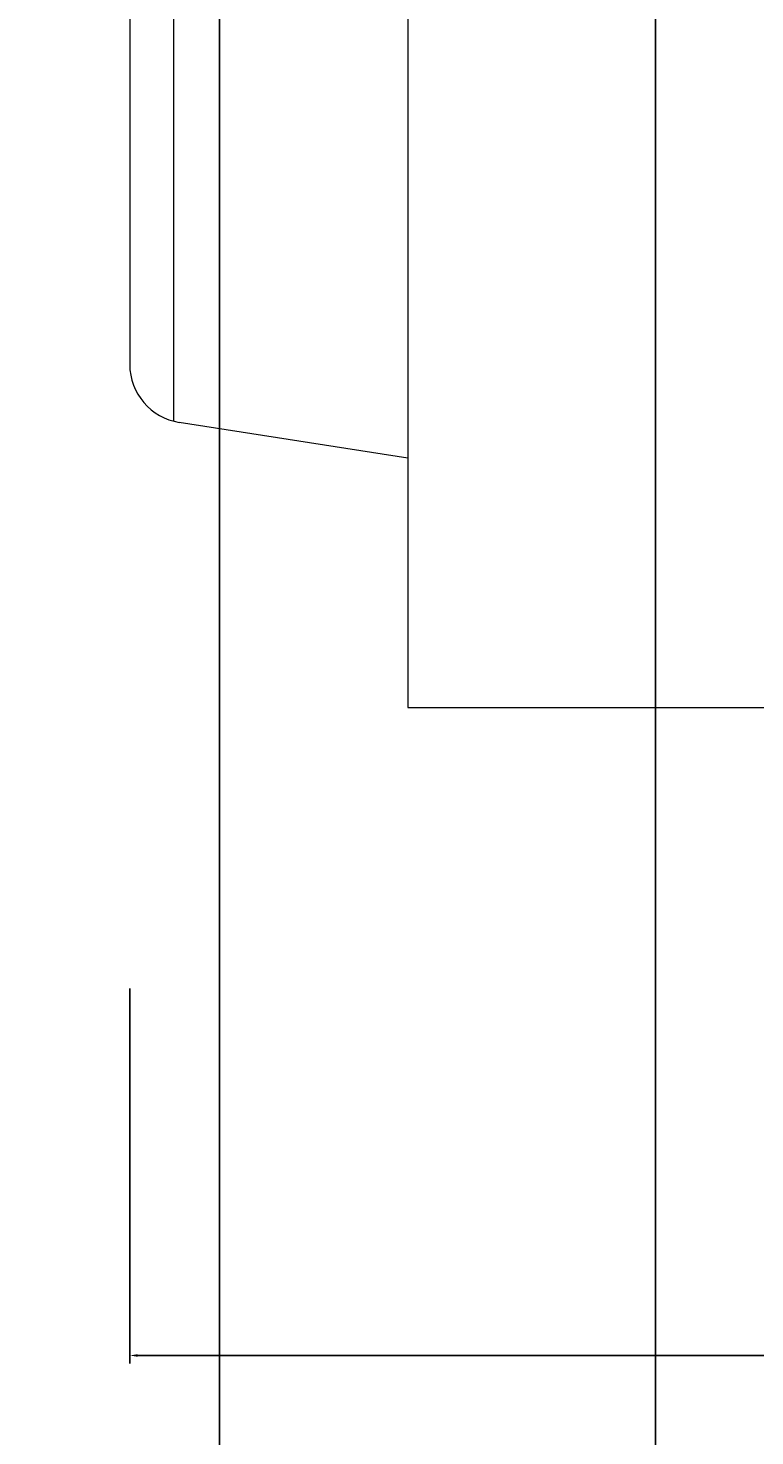
# Model space of a CAD drawing. Units: inches. Extents: x 2231 to 2461, y 2045 to 2455.
# Tile 23 of 95: x 2326 to 2343, y 2112 to 2144. Entities that reach past the tile are written whole.
import ezdxf

# ---------------------------------------------------------------- set-up
doc = ezdxf.new("R2010")
doc.units = ezdxf.units.IN
doc.layers.add('A-ANNO-DIMS', color=2, linetype='Continuous', lineweight=18)
doc.layers.add('A-FURN', color=9, linetype='Continuous', lineweight=18)
doc.styles.get("Standard").update_dxf_attribs({"font": 'arial.ttf'})
doc.dimstyles.get("Standard").update_dxf_attribs({"dimtxt": 0.18, "dimasz": 0.18, "dimexe": 0.18, "dimexo": 0.0625, "dimgap": 0.09, "dimtad": 0, "dimtih": 1, "dimtoh": 1, "dimdec": 4, "dimzin": 0, "dimdsep": 46, "dimtxsty": 'Standard', "dimcen": 0.09, "dimadec": 0, "dimazin": 0, "dimtfac": 1, "dimtdec": 4, "dimtofl": 0, "dimtmove": 0, "dimatfit": 3, "dimfxl": 1, "dimtolj": 1, "dimtzin": 0, "dimarcsym": 0})

# ---------------------------------------------------------------- blocks, each defined once
blk = doc.blocks.new('Dining Set - 36 x 72 in.')
for p, q in [((-36, 18), (-36, -18)), ((-44, 8.23), (-44, -8.239)), ((-45.5, 6.288), (-45.5, -6.288)), ((-35.998, -9.485), (-43.809, -8.264)), ((-36, -18), (-4.062, -18))]:
    blk.add_line(p, q)
blk.add_arc((-43.5, -6.288), 2, 180, 261.1194)
blk = doc.blocks.new('*D31')
at = {"layer": 'A-ANNO-DIMS', "color": 0, "lineweight": -2, "transparency": 16777216}
for p, q in [((2328.765, 2122.602), (2328.765, 2114.118)), ((2384.543, 2122.602), (2384.543, 2114.118)), ((2328.945, 2114.298), (2355.685, 2114.298)), ((2384.363, 2114.298), (2357.623, 2114.298))]:
    blk.add_line(p, q, dxfattribs=at)
at = {"layer": 'A-ANNO-DIMS', "color": 0, "transparency": 16777216}
for points in [[(2328.945, 2114.328), (2328.945, 2114.268), (2328.765, 2114.298)], [(2384.363, 2114.328), (2384.363, 2114.268), (2384.543, 2114.298)]]:
    blk.add_solid(points, dxfattribs=at)
at = {"layer": 'Defpoints', "color": 0, "transparency": 16777216}
for p in [(2328.765, 2122.665), (2384.543, 2122.665), (2384.543, 2114.298)]:
    blk.add_point(p, dxfattribs=at)
at = {"layer": 'A-ANNO-DIMS', "color": 0, "transparency": 16777216, "insert": (2356.654, 2114.298), "char_height": 0.18, "attachment_point": 5}
blk.add_mtext('\\A1;DINING SET 56', dxfattribs=at)
blk = doc.blocks.new('*D51')
at = {"layer": 'A-ANNO-DIMS', "color": 0, "lineweight": -2, "transparency": 16777216}
for p, q in [((2258.794, 2306.77), (2258.794, 2044.803)), ((2330.794, 2306.77), (2330.794, 2044.803)), ((2258.974, 2044.983), (2294.576, 2044.983)), ((2330.614, 2044.983), (2295.011, 2044.983))]:
    blk.add_line(p, q, dxfattribs=at)
at = {"layer": 'A-ANNO-DIMS', "color": 0, "transparency": 16777216}
for points in [[(2258.974, 2045.013), (2258.974, 2044.953), (2258.794, 2044.983)], [(2330.614, 2045.013), (2330.614, 2044.953), (2330.794, 2044.983)]]:
    blk.add_solid(points, dxfattribs=at)
at = {"layer": 'Defpoints', "color": 0, "transparency": 16777216}
for p in [(2258.794, 2306.833), (2330.794, 2306.833), (2330.794, 2044.983)]:
    blk.add_point(p, dxfattribs=at)
at = {"layer": 'A-ANNO-DIMS', "color": 0, "transparency": 16777216, "insert": (2294.794, 2044.983), "char_height": 0.18, "attachment_point": 5}
blk.add_mtext('\\A1;72', dxfattribs=at)
blk = doc.blocks.new('*D52')
at = {"layer": 'A-ANNO-DIMS', "color": 0, "lineweight": -2, "transparency": 16777216}
for p, q in [((2330.794, 2306.77), (2330.794, 2044.803)), ((2360.794, 2306.77), (2360.794, 2044.803)), ((2330.974, 2044.983), (2345.575, 2044.983)), ((2360.614, 2044.983), (2346.012, 2044.983))]:
    blk.add_line(p, q, dxfattribs=at)
at = {"layer": 'A-ANNO-DIMS', "color": 0, "transparency": 16777216}
for points in [[(2330.974, 2045.013), (2330.974, 2044.953), (2330.794, 2044.983)], [(2360.614, 2045.013), (2360.614, 2044.953), (2360.794, 2044.983)]]:
    blk.add_solid(points, dxfattribs=at)
at = {"layer": 'Defpoints', "color": 0, "transparency": 16777216}
for p in [(2330.794, 2306.833), (2360.794, 2306.833), (2360.794, 2044.983)]:
    blk.add_point(p, dxfattribs=at)
at = {"layer": 'A-ANNO-DIMS', "color": 0, "transparency": 16777216, "insert": (2345.794, 2044.983), "char_height": 0.18, "attachment_point": 5}
blk.add_mtext('\\A1;30', dxfattribs=at)
blk = doc.blocks.new('*D65')
at = {"layer": 'A-ANNO-DIMS', "color": 0, "lineweight": -2, "transparency": 16777216}
for p, q in [((2285.635, 2189.285), (2285.635, 2044.803)), ((2340.667, 2189.285), (2340.667, 2044.803)), ((2285.815, 2044.983), (2312.758, 2044.983)), ((2340.487, 2044.983), (2313.545, 2044.983))]:
    blk.add_line(p, q, dxfattribs=at)
at = {"layer": 'A-ANNO-DIMS', "color": 0, "transparency": 16777216}
for points in [[(2285.815, 2045.013), (2285.815, 2044.953), (2285.635, 2044.983)], [(2340.487, 2045.013), (2340.487, 2044.953), (2340.667, 2044.983)]]:
    blk.add_solid(points, dxfattribs=at)
at = {"layer": 'Defpoints', "color": 0, "transparency": 16777216}
for p in [(2285.635, 2189.348), (2340.667, 2189.348), (2340.667, 2044.983)]:
    blk.add_point(p, dxfattribs=at)
at = {"layer": 'A-ANNO-DIMS', "color": 0, "transparency": 16777216, "insert": (2313.151, 2044.983), "char_height": 0.18, "attachment_point": 5}
blk.add_mtext('\\A1;55.03', dxfattribs=at)
blk = doc.blocks.new('*D69')
at = {"layer": 'A-ANNO-DIMS', "color": 0, "lineweight": -2, "transparency": 16777216}
for p, q in [((2340.667, 2189.285), (2340.667, 2044.803)), ((2394.794, 2186.77), (2394.794, 2044.803)), ((2340.847, 2044.983), (2367.337, 2044.983)), ((2394.614, 2044.983), (2368.124, 2044.983))]:
    blk.add_line(p, q, dxfattribs=at)
at = {"layer": 'A-ANNO-DIMS', "color": 0, "transparency": 16777216}
for points in [[(2340.847, 2045.013), (2340.847, 2044.953), (2340.667, 2044.983)], [(2394.614, 2045.013), (2394.614, 2044.953), (2394.794, 2044.983)]]:
    blk.add_solid(points, dxfattribs=at)
at = {"layer": 'Defpoints', "color": 0, "transparency": 16777216}
for p in [(2340.667, 2189.348), (2394.794, 2186.833), (2394.794, 2044.983)]:
    blk.add_point(p, dxfattribs=at)
at = {"layer": 'A-ANNO-DIMS', "color": 0, "transparency": 16777216, "insert": (2367.73, 2044.983), "char_height": 0.18, "attachment_point": 5}
blk.add_mtext('\\A1;54.13', dxfattribs=at)

msp = doc.modelspace()

# ---------------------------------------------------------------- block references
at = {"layer": 'A-FURN', "xscale": 0.6627357546055535, "yscale": 0.6627357546055535, "zscale": 0.6627357546055535}
msp.add_blockref('Dining Set - 36 x 72 in.', (2358.9199, 2140.8902), dxfattribs=at)

# ---------------------------------------------------------------- dimensions: what is measured, and where the dimension line sits
at = {"layer": 'A-ANNO-DIMS'}
for base, p1, p2, override, picture, middle in [((2330.7935, 2044.9825), (2258.7935, 2306.8328), (2330.7935, 2306.8328), {"dimdec": 0, "dimlfac": 1, "dimrnd": 0, "dimzin": 0, "dimdsep": 46, "dimlunit": 2}, '*D51', (2294.7935, 2044.9825)), ((2360.7935, 2044.9825), (2330.7935, 2306.8328), (2360.7935, 2306.8328), {"dimdec": 0, "dimlfac": 1, "dimrnd": 0, "dimzin": 0, "dimdsep": 46, "dimlunit": 2}, '*D52', (2345.7935, 2044.9825)), ((2340.6673, 2044.9825), (2285.6353, 2189.3477), (2340.6673, 2189.3477), {"dimdec": 2, "dimlfac": 1, "dimrnd": 0, "dimzin": 0, "dimdsep": 46, "dimlunit": 2}, '*D65', (2313.1513, 2044.9825)), ((2394.7935, 2044.9825), (2340.6673, 2189.3477), (2394.7935, 2186.8328), {"dimdec": 2, "dimlfac": 1, "dimrnd": 0, "dimzin": 0, "dimdsep": 46, "dimlunit": 2}, '*D69', (2367.7304, 2044.9825))]:
    dim = msp.add_linear_dim(base=base, p1=p1, p2=p2, dimstyle='Standard', override=override, dxfattribs=at)
    dim.commit()
    dim.dimension.update_dxf_attribs({"geometry": picture, "text_midpoint": middle})
dim = msp.add_linear_dim(base=(2384.5428, 2114.2984), p1=(2328.7655, 2122.665), p2=(2384.5428, 2122.665), text='DINING SET <>', dimstyle='Standard', override={"dimdec": 0, "dimlfac": 1, "dimrnd": 0, "dimzin": 0, "dimdsep": 46, "dimlunit": 2}, dxfattribs=at)
dim.commit()
dim.dimension.update_dxf_attribs({"geometry": '*D31', "text_midpoint": (2356.6542, 2114.2984)})

doc.saveas('drawing.dxf')
